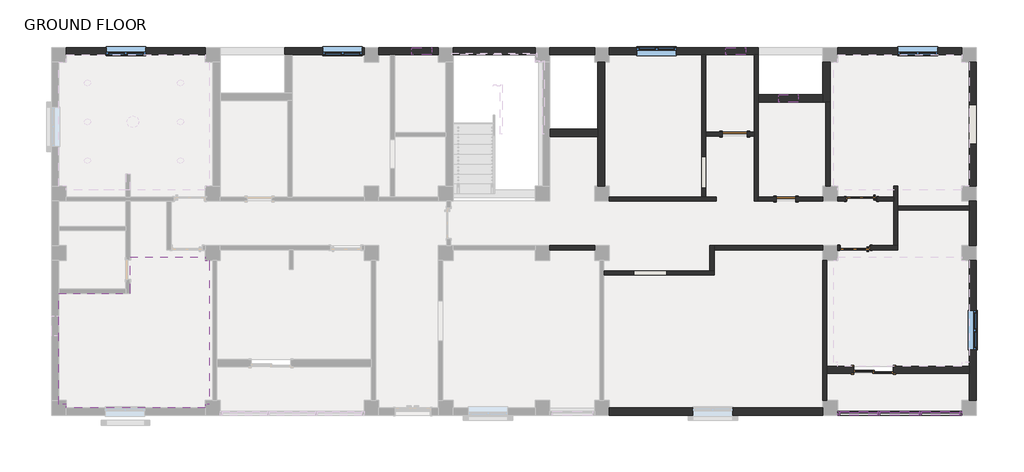
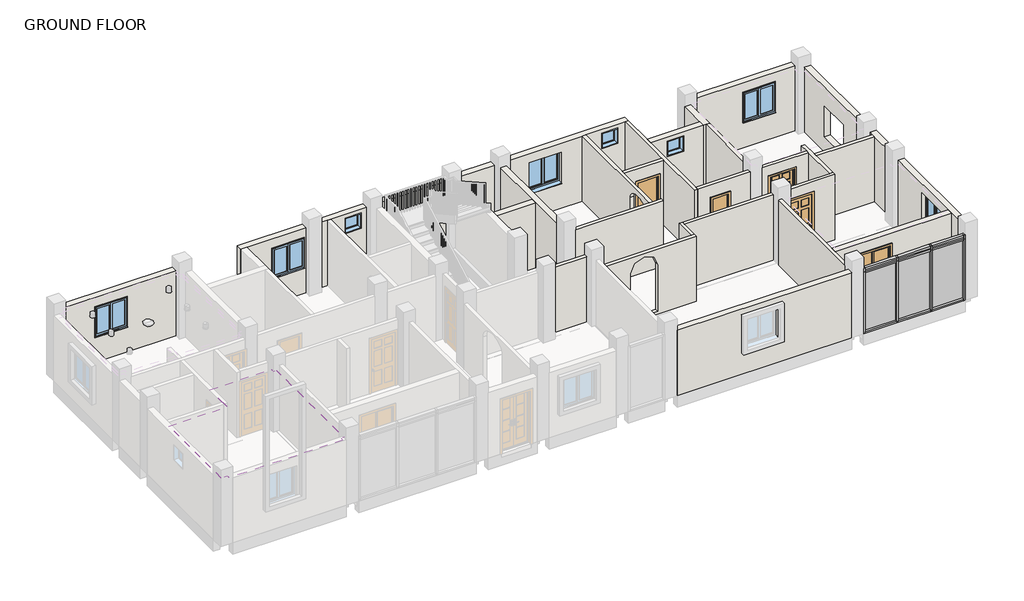
# One storey, part 2 of 5: 31 walls, 17 members, 8 windows, 6 plates, 5 doors, 1 covering.
"""IFC4 building model written with IfcOpenShell, lengths in millimetres."""

from ifc_helpers import new_model, si_unit, point, frame, origin, place, context, project, spatial, polyline, ellipse_curve, trimmed, outline, extrude, faceted_brep, transform, mapped, element, save
from ifc_brep_helpers import plane_surface, extruded_surface, advanced_brep
from components import door_double_sliding_4436dcad, door_c610b25b, door_03e3dfb5, single_flush_2_x_7_bath_room_door_025d1c86, door_1fe7f57d, member_5d96a33e, member_91edd790, member_f0fea5a5, member_f6f0dfdd, member_ee409385, member_876f8f00, member_7f2c8287, member_abd5b11f, system_panel_glazed_688a88ce, system_panel_glazed_153d3200, system_panel_glazed_8661f242, system_panel_glazed_4956db27, window_80340324, w2_0001_4_x_4_window_9dec5fc7

model = new_model("IFC4")

# Units and contexts
model_context = context("Model", 3, world=origin())
ifc_project = project(units=[si_unit("LENGTHUNIT", "METRE", prefix="MILLI")], contexts=[model_context])

# Site, building, storey
site = spatial("IfcSite", under=ifc_project)
building = spatial("IfcBuilding", under=site)
storey = spatial("IfcBuildingStorey", under=building, Name="GROUND FLOOR", Elevation=304.8)

# Covering
placement = place(None, origin())
element("IfcCovering", 1, ObjectType="GWB on Mtl. Stud", at=placement, inside=storey, context=model_context, shape_type="SweptSolid", body=[
    extrude(outline(polyline([(-15145.3456086, -10773.5679047), (-15145.3456086, -7363.1659448), (-12959.7401855, -7363.1659448), (-12959.7401855, -6244.0794704), (-10649.5456086, -6244.0794704), (-10649.5456086, -6358.3794704), (-10535.2456086, -6358.3794704), (-10535.2456086, -6963.5679047), (-10535.2456086, -10773.5679047), (-10649.5456086, -10773.5679047), (-10649.5456086, -10887.8679047), (-12959.7401855, -10887.8679047), (-14916.7456086, -10887.8679047), (-14916.7456086, -10773.5679047), (-15145.3456086, -10773.5679047)]), holes=[polyline([(-14840.5456086, -10583.0679047), (-10840.0456086, -10583.0679047), (-10840.0456086, -6548.8794704), (-12654.9401855, -6548.8794704), (-12654.9401855, -7667.9659448), (-14840.5456086, -7667.9659448), (-14840.5456086, -10583.0679047)])]), frame((0.0, 0.0, 2743.2), z_axis=(0.0, 0.0, 1.0), x_axis=(1.0, 0.0, 0.0)), (0.0, 0.0, 1.0), 107.95),
    extrude(outline(polyline([(-14688.1456086, -10430.6679047), (-14688.1456086, -7820.3659448), (-12502.5401855, -7820.3659448), (-12502.5401855, -6701.2794704), (-10992.4456086, -6701.2794704), (-10992.4456086, -10430.6679047), (-14688.1456086, -10430.6679047)]), holes=[polyline([(-14535.7456086, -7972.7659448), (-14535.7456086, -10278.2679047), (-11144.8456086, -10278.2679047), (-11144.8456086, -6853.6794704), (-12350.1401855, -6853.6794704), (-12350.1401855, -7972.7659448), (-14535.7456086, -7972.7659448)])]), frame((0.0, 0.0, 2743.2), z_axis=(0.0, 0.0, 1.0), x_axis=(1.0, 0.0, 0.0)), (0.0, 0.0, 1.0), 107.95),
])

# Doors
door_double_sliding_shape = door_double_sliding_4436dcad(model_context)
element("IfcDoor", 2, ObjectType="Door-Double-Sliding", at=placement, inside=storey, context=model_context, shape_type="MappedRepresentation", body=[
    mapped(door_double_sliding_shape, transform((9879.3128058, -9592.4679047, 304.8), x_axis=(-1.0, 0.0, 0.0), y_axis=(0.0, -1.0, 0.0), z_axis=(0.0, 0.0, 1.0))),
])
door_shape = door_c610b25b(model_context)
element("IfcDoor", 3, ObjectType="Door-Interior-Single-6_Panel-Wood : 36\" x 84\"", at=placement, inside=storey, context=model_context, shape_type="MappedRepresentation", body=[
    mapped(door_shape, transform((9511.0128058, -4462.9044704, 304.8), x_axis=(-1.0, 0.0, 0.0), y_axis=(0.0, -1.0, 0.0), z_axis=(0.0, 0.0, 1.0))),
])
door_2_shape = door_03e3dfb5(model_context)
element("IfcDoor", 4, ObjectType="Door-Interior-Single-6_Panel-Wood : 36\" x 84\"", at=placement, inside=storey, context=model_context, shape_type="MappedRepresentation", body=[
    mapped(door_2_shape, transform((9307.8128058, -5967.8544704, 304.8), x_axis=(-1.0, 0.0, 0.0), y_axis=(0.0, -1.0, 0.0), z_axis=(0.0, 0.0, 1.0))),
])
single_flush_2_x_7_bath_room_door_shape = single_flush_2_x_7_bath_room_door_025d1c86(model_context)
element("IfcDoor", 5, ObjectType="Single-Flush : 2' X 7' BATH ROOM DOOR", at=placement, inside=storey, context=model_context, shape_type="MappedRepresentation", body=[
    mapped(single_flush_2_x_7_bath_room_door_shape, transform((7190.4916602, -4466.0794704, 304.8), x_axis=(1.0, 0.0, 0.0), y_axis=(0.0, 1.0, 0.0), z_axis=(0.0, 0.0, 1.0))),
])
door_3_shape = door_1fe7f57d(model_context)
element("IfcDoor", 6, ObjectType="Single-Flush : 30\" x 80\"", at=placement, inside=storey, context=model_context, shape_type="MappedRepresentation", body=[
    mapped(door_3_shape, transform((5615.6916602, -2472.1794704, 304.8), x_axis=(1.0, 0.0, 0.0), y_axis=(0.0, 1.0, 0.0), z_axis=(0.0, 0.0, 1.0))),
])

# Members
member_shape = member_5d96a33e(model_context)
element("IfcMember", 7, ObjectType="Rectangular Mullion : 2.5\" x 5\" rectangular", at=placement, inside=storey, context=model_context, shape_type="MappedRepresentation", body=[
    mapped(member_shape, transform((12520.9128058, -11052.9679047, 2895.6), x_axis=(0.0, 0.0, 1.0), y_axis=(0.0, -1.0, 0.0), z_axis=(1.0, 0.0, 0.0))),
])
element("IfcMember", 8, ObjectType="Rectangular Mullion : 2.5\" x 5\" rectangular", at=placement, inside=storey, context=model_context, shape_type="MappedRepresentation", body=[
    mapped(member_shape, transform((10012.6628059, -11052.9679047, 2895.6), x_axis=(0.0, 0.0, 1.0), y_axis=(0.0, -1.0, 0.0), z_axis=(1.0, 0.0, 0.0))),
])
element("IfcMember", 9, ObjectType="Rectangular Mullion : 2.5\" x 5\" rectangular", at=placement, inside=storey, context=model_context, shape_type="MappedRepresentation", body=[
    mapped(member_shape, transform((8837.9128058, -11052.9679047, 304.8), x_axis=(0.0, 0.0, -1.0), y_axis=(0.0, -1.0, 0.0), z_axis=(-1.0, 0.0, 0.0))),
])
element("IfcMember", 10, ObjectType="Rectangular Mullion : 2.5\" x 5\" rectangular", at=placement, inside=storey, context=model_context, shape_type="MappedRepresentation", body=[
    mapped(member_shape, transform((11346.1628057, -11052.9679047, 304.8), x_axis=(0.0, 0.0, -1.0), y_axis=(0.0, -1.0, 0.0), z_axis=(-1.0, 0.0, 0.0))),
])
member_2_shape = member_91edd790(model_context)
element("IfcMember", 11, ObjectType="Rectangular Mullion : 2.5\" x 5\" rectangular", at=placement, inside=storey, context=model_context, shape_type="MappedRepresentation", body=[
    mapped(member_2_shape, transform((11282.6628057, -11052.9679047, 2895.6), x_axis=(0.0, 0.0, 1.0), y_axis=(0.0, -1.0, 0.0), z_axis=(1.0, 0.0, 0.0))),
])
element("IfcMember", 12, ObjectType="Rectangular Mullion : 2.5\" x 5\" rectangular", at=placement, inside=storey, context=model_context, shape_type="MappedRepresentation", body=[
    mapped(member_2_shape, transform((10076.1628059, -11052.9679047, 304.8), x_axis=(0.0, 0.0, -1.0), y_axis=(0.0, -1.0, 0.0), z_axis=(-1.0, 0.0, 0.0))),
])
member_3_shape = member_f0fea5a5(model_context)
element("IfcMember", 13, ObjectType="Rectangular Mullion : 2.5\" x 5\" rectangular", at=placement, inside=storey, context=model_context, shape_type="MappedRepresentation", body=[
    mapped(member_3_shape, transform((10044.4128059, -11052.9679047, 304.8), x_axis=(1.0, 0.0, 0.0), y_axis=(0.0, -1.0, 0.0), z_axis=(0.0, 0.0, -1.0))),
])
element("IfcMember", 14, ObjectType="Rectangular Mullion : 2.5\" x 5\" rectangular", at=placement, inside=storey, context=model_context, shape_type="MappedRepresentation", body=[
    mapped(member_3_shape, transform((11314.4128057, -11052.9679047, 304.8), x_axis=(1.0, 0.0, 0.0), y_axis=(0.0, -1.0, 0.0), z_axis=(0.0, 0.0, -1.0))),
])
member_4_shape = member_f6f0dfdd(model_context)
element("IfcMember", 15, ObjectType="Rectangular Mullion : 2.5\" x 5\" rectangular", at=placement, inside=storey, context=model_context, shape_type="MappedRepresentation", body=[
    mapped(member_4_shape, transform((10044.4128059, -11052.9679047, 2743.2), x_axis=(1.0, 0.0, 0.0), y_axis=(0.0, -1.0, 0.0), z_axis=(0.0, 0.0, -1.0))),
])
element("IfcMember", 16, ObjectType="Rectangular Mullion : 2.5\" x 5\" rectangular", at=placement, inside=storey, context=model_context, shape_type="MappedRepresentation", body=[
    mapped(member_4_shape, transform((11314.4128057, -11052.9679047, 2743.2), x_axis=(1.0, 0.0, 0.0), y_axis=(0.0, -1.0, 0.0), z_axis=(0.0, 0.0, -1.0))),
])
member_5_shape = member_ee409385(model_context)
element("IfcMember", 17, ObjectType="Rectangular Mullion : 2.5\" x 5\" rectangular", at=placement, inside=storey, context=model_context, shape_type="MappedRepresentation", body=[
    mapped(member_5_shape, transform((12584.4128058, -11052.9679047, 304.8), x_axis=(1.0, 0.0, 0.0), y_axis=(0.0, -1.0, 0.0), z_axis=(0.0, 0.0, -1.0))),
])
member_6_shape = member_876f8f00(model_context)
element("IfcMember", 18, ObjectType="Rectangular Mullion : 2.5\" x 5\" rectangular", at=placement, inside=storey, context=model_context, shape_type="MappedRepresentation", body=[
    mapped(member_6_shape, transform((8774.4128058, -11052.9679047, 2895.6), x_axis=(-1.0, 0.0, 0.0), y_axis=(0.0, -1.0, 0.0), z_axis=(0.0, 0.0, 1.0))),
])
element("IfcMember", 19, ObjectType="Rectangular Mullion : 2.5\" x 5\" rectangular", at=placement, inside=storey, context=model_context, shape_type="MappedRepresentation", body=[
    mapped(member_6_shape, transform((12584.4128058, -11052.9679047, 2743.2), x_axis=(1.0, 0.0, 0.0), y_axis=(0.0, -1.0, 0.0), z_axis=(0.0, 0.0, -1.0))),
])
element("IfcMember", 20, ObjectType="Rectangular Mullion : 2.5\" x 5\" rectangular", at=placement, inside=storey, context=model_context, shape_type="MappedRepresentation", body=[
    mapped(member_5_shape, transform((8774.4128058, -11052.9679047, 2743.2), x_axis=(-1.0, 0.0, 0.0), y_axis=(0.0, -1.0, 0.0), z_axis=(0.0, 0.0, 1.0))),
])
member_7_shape = member_7f2c8287(model_context)
element("IfcMember", 21, ObjectType="Rectangular Mullion : 2.5\" x 5\" rectangular", at=placement, inside=storey, context=model_context, shape_type="MappedRepresentation", body=[
    mapped(member_7_shape, transform((10012.6628059, -11052.9679047, 2743.2), x_axis=(0.0, 0.0, 1.0), y_axis=(0.0, -1.0, 0.0), z_axis=(1.0, 0.0, 0.0))),
])
element("IfcMember", 22, ObjectType="Rectangular Mullion : 2.5\" x 5\" rectangular", at=placement, inside=storey, context=model_context, shape_type="MappedRepresentation", body=[
    mapped(member_7_shape, transform((12520.9128058, -11052.9679047, 2743.2), x_axis=(0.0, 0.0, 1.0), y_axis=(0.0, -1.0, 0.0), z_axis=(1.0, 0.0, 0.0))),
])
member_8_shape = member_abd5b11f(model_context)
element("IfcMember", 23, ObjectType="Rectangular Mullion : 2.5\" x 5\" rectangular", at=placement, inside=storey, context=model_context, shape_type="MappedRepresentation", body=[
    mapped(member_8_shape, transform((11282.6628057, -11052.9679047, 2743.2), x_axis=(0.0, 0.0, 1.0), y_axis=(0.0, -1.0, 0.0), z_axis=(1.0, 0.0, 0.0))),
])

# Plates
system_panel_glazed_shape = system_panel_glazed_688a88ce(model_context)
element("IfcPlate", 24, ObjectType="System Panel : Glazed", at=placement, inside=storey, context=model_context, shape_type="MappedRepresentation", body=[
    mapped(system_panel_glazed_shape, transform((9425.2878058, -11052.9679047, 368.3), x_axis=(1.0, 0.0, 0.0), y_axis=(0.0, 1.0, 0.0), z_axis=(0.0, 0.0, 1.0))),
])
element("IfcPlate", 25, ObjectType="System Panel : Glazed", at=placement, inside=storey, context=model_context, shape_type="MappedRepresentation", body=[
    mapped(system_panel_glazed_shape, transform((11933.5378057, -11052.9679047, 368.3), x_axis=(1.0, 0.0, 0.0), y_axis=(0.0, 1.0, 0.0), z_axis=(0.0, 0.0, 1.0))),
])
system_panel_glazed_2_shape = system_panel_glazed_153d3200(model_context)
element("IfcPlate", 26, ObjectType="System Panel : Glazed", at=placement, inside=storey, context=model_context, shape_type="MappedRepresentation", body=[
    mapped(system_panel_glazed_2_shape, transform((10679.4128058, -11052.9679047, 368.3), x_axis=(1.0, 0.0, 0.0), y_axis=(0.0, 1.0, 0.0), z_axis=(0.0, 0.0, 1.0))),
])
system_panel_glazed_3_shape = system_panel_glazed_8661f242(model_context)
element("IfcPlate", 27, ObjectType="System Panel : Glazed", at=placement, inside=storey, context=model_context, shape_type="MappedRepresentation", body=[
    mapped(system_panel_glazed_3_shape, transform((9425.2878058, -11052.9679047, 2774.95), x_axis=(1.0, 0.0, 0.0), y_axis=(0.0, 1.0, 0.0), z_axis=(0.0, 0.0, 1.0))),
])
element("IfcPlate", 28, ObjectType="System Panel : Glazed", at=placement, inside=storey, context=model_context, shape_type="MappedRepresentation", body=[
    mapped(system_panel_glazed_3_shape, transform((11933.5378057, -11052.9679047, 2774.95), x_axis=(1.0, 0.0, 0.0), y_axis=(0.0, 1.0, 0.0), z_axis=(0.0, 0.0, 1.0))),
])
system_panel_glazed_4_shape = system_panel_glazed_4956db27(model_context)
element("IfcPlate", 29, ObjectType="System Panel : Glazed", at=placement, inside=storey, context=model_context, shape_type="MappedRepresentation", body=[
    mapped(system_panel_glazed_4_shape, transform((10679.4128058, -11052.9679047, 2774.95), x_axis=(1.0, 0.0, 0.0), y_axis=(0.0, 1.0, 0.0), z_axis=(0.0, 0.0, 1.0))),
])

# Walls
element("IfcWall", 30, ObjectType="EXTERIOR WALL 9\"", at=placement, inside=storey, context=model_context, shape_type="SweptSolid", body=[
    extrude(outline(polyline([(304.8, 1767.5916602), (304.8, 8317.2128058), (2895.6, 8317.2128058), (2895.6, 1767.5916602), (304.8, 1767.5916602)]), holes=[polyline([(1304.8, 5552.1916602), (1304.8, 4332.9916602), (2524.0, 4332.9916602), (2524.0, 5552.1916602), (1304.8, 5552.1916602)])]), frame((0.0, -11116.4679047, 0.0), z_axis=(0.0, 1.0, 0.0), x_axis=(0.0, 0.0, 1.0)), (0.0, 0.0, 1.0), 228.6),
])
element("IfcWall", 31, ObjectType="EXTERIOR WALL 9\"", at=placement, inside=storey, context=model_context, shape_type="Brep", body=[
    faceted_brep([(13041.6128058, -10659.2679047, 304.8), (13041.6128058, -6358.3794704, 304.8), (13041.6128058, -6358.3794704, 2895.6), (13041.6128058, -10659.2679047, 2895.6), (13041.6128058, -9109.8679047, 1304.8), (13041.6128058, -9109.8679047, 2524.0), (13041.6128058, -7890.6679047, 2524.0), (13041.6128058, -7890.6679047, 1304.8), (12813.0128058, -10659.2679047, 304.8), (12813.0128058, -10659.2679047, 2895.6), (12813.0128058, -9833.7679047, 2895.6), (12813.0128058, -9605.1679047, 2895.6), (12813.0128058, -6358.3794704, 2895.6), (12813.0128058, -6358.3794704, 304.8), (12813.0128058, -9605.1679047, 304.8), (12813.0128058, -9833.7679047, 304.8), (12813.0128058, -9109.8679047, 1304.8), (12813.0128058, -7890.6679047, 1304.8), (12813.0128058, -7890.6679047, 2524.0), (12813.0128058, -9109.8679047, 2524.0)], [[[0, 1, 2, 3], [4, 5, 6, 7]], [[8, 9, 10, 11, 12, 13, 14, 15], [16, 17, 18, 19]], [[1, 0, 8, 15, 14, 13]], [[2, 1, 13, 12]], [[3, 2, 12, 11, 10, 9]], [[0, 3, 9, 8]], [[5, 4, 16, 19]], [[6, 5, 19, 18]], [[7, 6, 18, 17]], [[4, 7, 17, 16]]]),
])
element("IfcWall", 32, ObjectType="EXTERIOR WALL 9\"", at=placement, inside=storey, context=model_context, shape_type="Brep", body=[
    faceted_brep([(13041.6128058, -5901.1794704, 304.8), (13041.6128058, -4529.5794704, 304.8), (13041.6128058, -4529.5794704, 2895.6), (13041.6128058, -5901.1794704, 2895.6), (12813.0128058, -5901.1794704, 304.8), (12813.0128058, -5901.1794704, 2895.6), (12813.0128058, -4808.9794704, 2895.6), (12813.0128058, -4681.9794704, 2895.6), (12813.0128058, -4529.5794704, 2895.6), (12813.0128058, -4529.5794704, 304.8), (12813.0128058, -4681.9794704, 304.8), (12813.0128058, -4808.9794704, 304.8)], [[[0, 1, 2, 3]], [[4, 5, 6, 7, 8, 9, 10, 11]], [[1, 0, 4, 11, 10, 9]], [[2, 1, 9, 8]], [[3, 2, 8, 7, 6, 5]], [[0, 3, 5, 4]]]),
])
element("IfcWall", 33, ObjectType="EXTERIOR WALL 9\"", at=placement, inside=storey, context=model_context, shape_type="SweptSolid", body=[
    extrude(outline(polyline([(-4072.3794704, 304.8), (-4072.3794704, 2895.6), (-262.3794704, 2895.6), (-262.3794704, 304.8), (-4072.3794704, 304.8)]), holes=[polyline([(-2776.9794704, 914.4), (-1557.7794704, 914.4), (-1557.7794704, 2133.6), (-2776.9794704, 2133.6), (-2776.9794704, 914.4)])]), frame((12813.0128058, 0.0, 0.0), z_axis=(1.0, 0.0, 0.0), x_axis=(0.0, 1.0, 0.0)), (0.0, 0.0, 1.0), 228.6),
])
element("IfcWall", 34, ObjectType="EXTERIOR WALL 9\"", at=placement, inside=storey, context=model_context, shape_type="SweptSolid", body=[
    extrude(outline(polyline([(304.8, 12584.4128058), (2895.6, 12584.4128058), (2895.6, 8774.4128058), (304.8, 8774.4128058), (304.8, 12584.4128058)]), holes=[polyline([(1304.8, 10628.6128058), (2524.0, 10628.6128058), (2524.0, 11847.8128058), (1304.8, 11847.8128058), (1304.8, 10628.6128058)])]), frame((0.0, -33.7794704, 0.0), z_axis=(0.0, 1.0, 0.0), x_axis=(0.0, 0.0, 1.0)), (0.0, 0.0, 1.0), 228.6),
])
element("IfcWall", 35, ObjectType="EXTERIOR WALL 9\"", at=placement, inside=storey, context=model_context, shape_type="SweptSolid", body=[
    extrude(outline(polyline([(304.8, -14916.7456086), (304.8, -10649.5456086), (2895.6, -10649.5456086), (2895.6, -14916.7456086), (304.8, -14916.7456086)]), holes=[polyline([(1304.8, -13697.5456086), (2524.0, -13697.5456086), (2524.0, -12478.3456086), (1304.8, -12478.3456086), (1304.8, -13697.5456086)])]), frame((0.0, -33.7794704, 0.0), z_axis=(0.0, 1.0, 0.0), x_axis=(0.0, 0.0, 1.0)), (0.0, 0.0, 1.0), 228.6),
])
element("IfcWall", 36, ObjectType="EXTERIOR WALL 9\"", at=placement, inside=storey, context=model_context, shape_type="SweptSolid", body=[
    extrude(outline(polyline([(304.8, 8444.2128058), (304.8, 9269.7128058), (2438.4, 9269.7128058), (2438.4, 10488.9128058), (304.8, 10488.9128058), (304.8, 12813.0128058), (2895.6, 12813.0128058), (2895.6, 8444.2128058), (304.8, 8444.2128058)])), frame((0.0, -9833.7679047, 0.0), z_axis=(0.0, 1.0, 0.0), x_axis=(0.0, 0.0, 1.0)), (0.0, 0.0, 1.0), 228.6),
])
element("IfcWall", 37, ObjectType="EXTERIOR WALL 9\"", at=placement, inside=storey, context=model_context, shape_type="Brep", body=[
    faceted_brep([(-5772.7456086, 194.8205296, 304.8), (-8211.1456086, 194.8205296, 304.8), (-8211.1456086, 194.8205296, 2895.6), (-5772.7456086, 194.8205296, 2895.6), (-7042.7456086, 194.8205296, 1304.8), (-5823.5456086, 194.8205296, 1304.8), (-5823.5456086, 194.8205296, 2524.0), (-7042.7456086, 194.8205296, 2524.0), (-5772.7456086, -33.7794704, 304.8), (-5772.7456086, -33.7794704, 2895.6), (-7982.5456086, -33.7794704, 2895.6), (-8211.1456086, -33.7794704, 2895.6), (-8211.1456086, -33.7794704, 304.8), (-7982.5456086, -33.7794704, 304.8), (-7042.7456086, -33.7794704, 1304.8), (-7042.7456086, -33.7794704, 2524.0), (-5823.5456086, -33.7794704, 2524.0), (-5823.5456086, -33.7794704, 1304.8)], [[[0, 1, 2, 3], [4, 5, 6, 7]], [[8, 9, 10, 11, 12, 13], [14, 15, 16, 17]], [[1, 0, 8, 13, 12]], [[3, 2, 11, 10, 9]], [[0, 3, 9, 8]], [[2, 1, 12, 11]], [[15, 14, 4, 7]], [[16, 15, 7, 6]], [[17, 16, 6, 5]], [[14, 17, 5, 4]]]),
])
element("IfcWall", 38, ObjectType="EXTERIOR WALL 9\"", at=placement, inside=storey, context=model_context, shape_type="Brep", body=[
    faceted_brep([(-5315.5456086, -33.7794704, 304.8), (-4959.9456086, -33.7794704, 304.8), (-4832.9456086, -33.7794704, 304.8), (-3486.7456086, -33.7794704, 304.8), (-3486.7456086, -33.7794704, 2895.6), (-4832.9456086, -33.7794704, 2895.6), (-4959.9456086, -33.7794704, 2895.6), (-5315.5456086, -33.7794704, 2895.6), (-3689.9456086, -33.7794704, 2743.2), (-3689.9456086, -33.7794704, 2133.6), (-4299.5456086, -33.7794704, 2133.6), (-4299.5456086, -33.7794704, 2743.2), (-3486.7456086, 194.8205296, 304.8), (-5315.5456086, 194.8205296, 304.8), (-5315.5456086, 194.8205296, 2895.6), (-3486.7456086, 194.8205296, 2895.6), (-3689.9456086, 194.8205296, 2133.6), (-3689.9456086, 194.8205296, 2743.2), (-4299.5456086, 194.8205296, 2743.2), (-4299.5456086, 194.8205296, 2133.6)], [[[0, 1, 2, 3, 4, 5, 6, 7], [8, 9, 10, 11]], [[12, 13, 14, 15], [16, 17, 18, 19]], [[3, 2, 1, 0, 13, 12]], [[4, 3, 12, 15]], [[7, 6, 5, 4, 15, 14]], [[0, 7, 14, 13]], [[8, 17, 16, 9]], [[9, 16, 19, 10]], [[10, 19, 18, 11]], [[17, 8, 11, 18]]]),
])
element("IfcWall", 39, ObjectType="EXTERIOR WALL 9\"", at=placement, inside=storey, context=model_context, shape_type="SweptSolid", body=[
    extrude(outline(polyline([(-518.4083398, -33.7794704), (-3029.5456086, -33.7794704), (-3029.5456086, 194.8205296), (-518.4083398, 194.8205296), (-518.4083398, -33.7794704)])), frame((0.0, 0.0, 304.8), z_axis=(0.0, 0.0, 1.0), x_axis=(1.0, 0.0, 0.0)), (0.0, 0.0, 1.0), 2590.8),
])
element("IfcWall", 40, ObjectType="EXTERIOR WALL 9\"", at=placement, inside=storey, context=model_context, shape_type="SweptSolid", body=[
    extrude(outline(polyline([(1310.3916602, -33.7794704), (-61.2083398, -33.7794704), (-61.2083398, 194.8205296), (1310.3916602, 194.8205296), (1310.3916602, -33.7794704)])), frame((0.0, 0.0, 304.8), z_axis=(0.0, 0.0, 1.0), x_axis=(1.0, 0.0, 0.0)), (0.0, 0.0, 1.0), 2590.8),
])
element("IfcWall", 41, ObjectType="EXTERIOR WALL 9\"", at=placement, inside=storey, context=model_context, shape_type="Brep", body=[
    faceted_brep([(1767.5916602, -33.7794704, 304.8), (4599.6916602, -33.7794704, 304.8), (4726.6916602, -33.7794704, 304.8), (6212.5916602, -33.7794704, 304.8), (6339.5916602, -33.7794704, 304.8), (6339.5916602, -33.7794704, 2895.6), (6212.5916602, -33.7794704, 2895.6), (4726.6916602, -33.7794704, 2895.6), (4599.6916602, -33.7794704, 2895.6), (1767.5916602, -33.7794704, 2895.6), (3824.9916602, -33.7794704, 1304.8), (2605.7916602, -33.7794704, 1304.8), (2605.7916602, -33.7794704, 2524.0), (3824.9916602, -33.7794704, 2524.0), (5945.8916602, -33.7794704, 2743.2), (5945.8916602, -33.7794704, 2133.6), (5336.2916602, -33.7794704, 2133.6), (5336.2916602, -33.7794704, 2743.2), (6339.5916602, 194.8205296, 304.8), (1767.5916602, 194.8205296, 304.8), (1767.5916602, 194.8205296, 2895.6), (6339.5916602, 194.8205296, 2895.6), (3824.9916602, 194.8205296, 1304.8), (3824.9916602, 194.8205296, 2524.0), (2605.7916602, 194.8205296, 2524.0), (2605.7916602, 194.8205296, 1304.8), (5945.8916602, 194.8205296, 2133.6), (5945.8916602, 194.8205296, 2743.2), (5336.2916602, 194.8205296, 2743.2), (5336.2916602, 194.8205296, 2133.6)], [[[0, 1, 2, 3, 4, 5, 6, 7, 8, 9], [10, 11, 12, 13], [14, 15, 16, 17]], [[18, 19, 20, 21], [22, 23, 24, 25], [26, 27, 28, 29]], [[4, 3, 2, 1, 0, 19, 18]], [[9, 8, 7, 6, 5, 21, 20]], [[0, 9, 20, 19]], [[5, 4, 18, 21]], [[23, 22, 10, 13]], [[24, 23, 13, 12]], [[25, 24, 12, 11]], [[22, 25, 11, 10]], [[14, 27, 26, 15]], [[15, 26, 29, 16]], [[16, 29, 28, 17]], [[27, 14, 17, 28]]]),
])
element("IfcWall", 42, ObjectType="EXTERIOR WALL 9\"", at=placement, inside=storey, context=model_context, shape_type="Brep", body=[
    faceted_brep([(8317.2128058, -262.3794704, 304.8), (8317.2128058, -1252.9794704, 304.8), (8317.2128058, -1481.5794704, 304.8), (8317.2128058, -1481.5794704, 2895.6), (8317.2128058, -1252.9794704, 2895.6), (8317.2128058, -262.3794704, 2895.6), (8545.8128058, -262.3794704, 304.8), (8545.8128058, -262.3794704, 2895.6), (8545.8128058, -1481.5794704, 2895.6), (8545.8128058, -1481.5794704, 304.8), (8418.8128058, -1481.5794704, 304.8), (8418.8128058, -1481.5794704, 2895.6)], [[[0, 1, 2, 3, 4, 5]], [[6, 7, 8, 9]], [[2, 1, 0, 6, 9, 10]], [[5, 4, 3, 11, 8, 7]], [[0, 5, 7, 6]], [[3, 2, 10, 9, 8, 11]]]),
])
element("IfcWall", 43, ObjectType="EXTERIOR WALL 9\"", at=placement, inside=storey, context=model_context, shape_type="SweptSolid", body=[
    extrude(outline(polyline([(304.8, 6339.5916602), (304.8, 8317.2128058), (2895.6, 8317.2128058), (2895.6, 6339.5916602), (304.8, 6339.5916602)]), holes=[polyline([(2743.2, 7571.4916602), (2133.6, 7571.4916602), (2133.6, 6961.8916602), (2743.2, 6961.8916602), (2743.2, 7571.4916602)])]), frame((0.0, -1481.5794704, 0.0), z_axis=(0.0, 1.0, 0.0), x_axis=(0.0, 0.0, 1.0)), (0.0, 0.0, 1.0), 228.6),
])
element("IfcWall", 44, ObjectType="EXTERIOR WALL 9\"", at=placement, inside=storey, context=model_context, shape_type="Brep", body=[
    faceted_brep([(1399.2916602, -262.3794704, 304.8), (1399.2916602, -2319.7794704, 304.8), (1399.2916602, -2548.3794704, 304.8), (1399.2916602, -4072.3794704, 304.8), (1399.2916602, -4072.3794704, 2895.6), (1399.2916602, -2548.3794704, 2895.6), (1399.2916602, -2319.7794704, 2895.6), (1399.2916602, -262.3794704, 2895.6), (1627.8916602, -262.3794704, 304.8), (1627.8916602, -262.3794704, 2895.6), (1627.8916602, -4072.3794704, 2895.6), (1627.8916602, -4072.3794704, 304.8)], [[[0, 1, 2, 3, 4, 5, 6, 7]], [[8, 9, 10, 11]], [[3, 2, 1, 0, 8, 11]], [[4, 3, 11, 10]], [[7, 6, 5, 4, 10, 9]], [[0, 7, 9, 8]]]),
])
element("IfcWall", 45, ObjectType="EXTERIOR WALL 9\"", at=placement, inside=storey, context=model_context, shape_type="SweptSolid", body=[
    extrude(outline(polyline([(1399.2916602, -2548.3794704), (-61.2083398, -2548.3794704), (-61.2083398, -2319.7794704), (1399.2916602, -2319.7794704), (1399.2916602, -2548.3794704)])), frame((0.0, 0.0, 304.8), z_axis=(0.0, 0.0, 1.0), x_axis=(1.0, 0.0, 0.0)), (0.0, 0.0, 1.0), 2590.8),
])
element("IfcWall", 46, ObjectType="INTERIOR WALL 5\"", at=placement, inside=storey, context=model_context, shape_type="Brep", body=[
    faceted_brep([(8444.2128058, -10659.2679047, 304.8), (8444.2128058, -9833.7679047, 304.8), (8444.2128058, -9605.1679047, 304.8), (8444.2128058, -6358.3794704, 304.8), (8444.2128058, -6358.3794704, 2895.6), (8444.2128058, -9605.1679047, 2895.6), (8444.2128058, -9833.7679047, 2895.6), (8444.2128058, -10659.2679047, 2895.6), (8317.2128058, -10659.2679047, 304.8), (8317.2128058, -10659.2679047, 2895.6), (8317.2128058, -6358.3794704, 2895.6), (8317.2128058, -6358.3794704, 304.8)], [[[0, 1, 2, 3, 4, 5, 6, 7]], [[8, 9, 10, 11]], [[3, 2, 1, 0, 8, 11]], [[4, 3, 11, 10]], [[7, 6, 5, 4, 10, 9]], [[0, 7, 9, 8]]]),
])
element("IfcWall", 47, ObjectType="INTERIOR WALL 5\"", at=placement, inside=storey, context=model_context, shape_type="SweptSolid", body=[
    extrude(outline(polyline([(10628.6128058, -4681.9794704), (12813.0128058, -4681.9794704), (12813.0128058, -4808.9794704), (10628.6128058, -4808.9794704), (10628.6128058, -4681.9794704)])), frame((0.0, 0.0, 304.8), z_axis=(0.0, 0.0, 1.0), x_axis=(1.0, 0.0, 0.0)), (0.0, 0.0, 1.0), 2590.8),
])
element("IfcWall", 48, ObjectType="INTERIOR WALL 5\"", at=placement, inside=storey, context=model_context, shape_type="Brep", body=[
    faceted_brep([(10628.6128058, -6028.1794704, 2895.6), (8774.4128058, -6028.1794704, 2895.6), (8774.4128058, -6028.1794704, 304.8), (8825.2128058, -6028.1794704, 304.8), (8825.2128058, -6028.1794704, 2463.8), (9790.4128058, -6028.1794704, 2463.8), (9790.4128058, -6028.1794704, 304.8), (10628.6128058, -6028.1794704, 304.8), (8774.4128058, -5901.1794704, 2895.6), (10501.6128058, -5901.1794704, 2895.6), (10628.6128058, -5901.1794704, 2895.6), (10628.6128058, -5901.1794704, 304.8), (10501.6128058, -5901.1794704, 304.8), (9790.4128058, -5901.1794704, 304.8), (9790.4128058, -5901.1794704, 2463.8), (8825.2128058, -5901.1794704, 2463.8), (8825.2128058, -5901.1794704, 304.8), (8774.4128058, -5901.1794704, 304.8)], [[[0, 1, 2, 3, 4, 5, 6, 7]], [[8, 9, 10, 11, 12, 13, 14, 15, 16, 17]], [[2, 17, 16, 3]], [[11, 7, 6, 13, 12]], [[1, 0, 10, 9, 8]], [[2, 1, 8, 17]], [[0, 7, 11, 10]], [[15, 4, 3, 16]], [[4, 15, 14, 5]], [[5, 14, 13, 6]]]),
])
element("IfcWall", 49, ObjectType="INTERIOR WALL 5\"", at=placement, inside=storey, context=model_context, shape_type="Brep", body=[
    faceted_brep([(10628.6128058, -5901.1794704, 304.8), (10628.6128058, -4808.9794704, 304.8), (10628.6128058, -4681.9794704, 304.8), (10628.6128058, -4072.3794704, 304.8), (10628.6128058, -4072.3794704, 2895.6), (10628.6128058, -4681.9794704, 2895.6), (10628.6128058, -4808.9794704, 2895.6), (10628.6128058, -5901.1794704, 2895.6), (10501.6128058, -5901.1794704, 304.8), (10501.6128058, -5901.1794704, 2895.6), (10501.6128058, -4529.5794704, 2895.6), (10501.6128058, -4402.5794704, 2895.6), (10501.6128058, -4072.3794704, 2895.6), (10501.6128058, -4072.3794704, 304.8), (10501.6128058, -4402.5794704, 304.8), (10501.6128058, -4529.5794704, 304.8)], [[[0, 1, 2, 3, 4, 5, 6, 7]], [[8, 9, 10, 11, 12, 13, 14, 15]], [[3, 2, 1, 0, 8, 15, 14, 13]], [[4, 3, 13, 12]], [[7, 6, 5, 4, 12, 11, 10, 9]], [[0, 7, 9, 8]]]),
])
element("IfcWall", 50, ObjectType="INTERIOR WALL 5\"", at=placement, inside=storey, context=model_context, shape_type="Brep", body=[
    faceted_brep([(6212.5916602, -33.7794704, 304.8), (6212.5916602, -2408.6794704, 304.8), (6212.5916602, -2535.6794704, 304.8), (6212.5916602, -4529.5794704, 304.8), (6212.5916602, -4529.5794704, 2895.6), (6212.5916602, -2535.6794704, 2895.6), (6212.5916602, -2408.6794704, 2895.6), (6212.5916602, -33.7794704, 2895.6), (6339.5916602, -33.7794704, 304.8), (6339.5916602, -33.7794704, 2895.6), (6339.5916602, -1252.9794704, 2895.6), (6339.5916602, -1481.5794704, 2895.6), (6339.5916602, -4402.5794704, 2895.6), (6339.5916602, -4529.5794704, 2895.6), (6339.5916602, -4529.5794704, 304.8), (6339.5916602, -4402.5794704, 304.8), (6339.5916602, -1481.5794704, 304.8), (6339.5916602, -1252.9794704, 304.8)], [[[0, 1, 2, 3, 4, 5, 6, 7]], [[8, 9, 10, 11, 12, 13, 14, 15, 16, 17]], [[3, 2, 1, 0, 8, 17, 16, 15, 14]], [[7, 6, 5, 4, 13, 12, 11, 10, 9]], [[0, 7, 9, 8]], [[4, 3, 14, 13]]]),
])
element("IfcWall", 51, ObjectType="INTERIOR WALL 5\"", at=placement, inside=storey, context=model_context, shape_type="SweptSolid", body=[
    extrude(outline(polyline([(8418.8128058, -4072.3794704), (8418.8128058, -1481.5794704), (8545.8128058, -1481.5794704), (8545.8128058, -4072.3794704), (8418.8128058, -4072.3794704)])), frame((0.0, 0.0, 304.8), z_axis=(0.0, 0.0, 1.0), x_axis=(1.0, 0.0, 0.0)), (0.0, 0.0, 1.0), 2590.8),
])
element("IfcWall", 52, ObjectType="INTERIOR WALL 5\"", at=placement, inside=storey, context=model_context, shape_type="Brep", body=[
    faceted_brep([(1767.5916602, -4529.5794704, 304.8), (5044.1916602, -4529.5794704, 304.8), (5044.1916602, -4529.5794704, 2895.6), (1767.5916602, -4529.5794704, 2895.6), (1767.5916602, -4402.5794704, 304.8), (1767.5916602, -4402.5794704, 2895.6), (4599.6916602, -4402.5794704, 2895.6), (4726.6916602, -4402.5794704, 2895.6), (5044.1916602, -4402.5794704, 2895.6), (5044.1916602, -4402.5794704, 304.8), (4726.6916602, -4402.5794704, 304.8), (4599.6916602, -4402.5794704, 304.8)], [[[0, 1, 2, 3]], [[4, 5, 6, 7, 8, 9, 10, 11]], [[1, 0, 4, 11, 10, 9]], [[2, 1, 9, 8]], [[3, 2, 8, 7, 6, 5]], [[0, 3, 5, 4]]]),
])
element("IfcWall", 53, ObjectType="INTERIOR WALL 5\"", at=placement, inside=storey, context=model_context, shape_type="AdvancedBrep", body=[
    advanced_brep(
    [(4599.6916602, -33.7794704, 304.8), (4599.6916602, -4402.5794704, 304.8), (4599.6916602, -4402.5794704, 2895.6), (4599.6916602, -33.7794704, 2895.6), (4599.6916602, -3162.9760679, 2363.4701015), (4599.6916602, -4128.1760679, 2363.4701015), (4599.6916602, -4128.1760679, 483.8701015), (4599.6916602, -3162.9760679, 483.8701015), (4726.6916602, -33.7794704, 304.8), (4726.6916602, -33.7794704, 2895.6), (4726.6916602, -2408.6794704, 2895.6), (4726.6916602, -2535.6794704, 2895.6), (4726.6916602, -4402.5794704, 2895.6), (4726.6916602, -4402.5794704, 304.8), (4726.6916602, -2535.6794704, 304.8), (4726.6916602, -2408.6794704, 304.8), (4726.6916602, -3162.9760679, 2363.4701015), (4726.6916602, -3162.9760679, 483.8701015), (4726.6916602, -4128.1760679, 483.8701015), (4726.6916602, -4128.1760679, 2363.4701015)],
    [
        (0, 1),
        (1, 2),
        (2, 3),
        (3, 0),
        (4, 5, ellipse_curve(frame((4599.6916602, -3645.5760679, 2363.4701015), z_axis=(1.0, 0.0, 0.0), x_axis=(0.0, -1.0, 0.0)), 482.6, 330.2)),
        (5, 6),
        (6, 7),
        (7, 4),
        (8, 9),
        (9, 10),
        (10, 11),
        (11, 12),
        (12, 13),
        (13, 14),
        (14, 15),
        (15, 8),
        (16, 17),
        (17, 18),
        (18, 19),
        (19, 16, ellipse_curve(frame((4726.6916602, -3645.5760679, 2363.4701015), z_axis=(-1.0, 0.0, 0.0), x_axis=(0.0, -1.0, 0.0)), 482.6, 330.2)),
        (3, 9),
        (8, 0),
        (1, 13),
        (12, 2),
        (4, 16),
        (19, 5),
        (18, 6),
        (17, 7),
    ],
    [
        plane_surface(frame((4599.6916602, -33.7794704, 304.8), z_axis=(-1.0, 0.0, 0.0), x_axis=(0.0, -1.0, 0.0))),
        plane_surface(frame((4726.6916602, -33.7794704, 304.8), z_axis=(1.0, 0.0, 0.0), x_axis=(0.0, 1.0, 0.0))),
        plane_surface(frame((1784.6412895, -33.7794704, 304.8), z_axis=(0.0, 1.0, 0.0), x_axis=(1.0, 0.0, 0.0))),
        plane_surface(frame((1767.5916602, -4402.5794704, 304.8), z_axis=(0.0, -1.0, 0.0), x_axis=(-1.0, 0.0, 0.0))),
        plane_surface(frame((4599.6916602, 80.5205296, 304.8), z_axis=(0.0, 0.0, -1.0), x_axis=(1.0, 0.0, 0.0))),
        plane_surface(frame((4599.6916602, -4466.0794704, 2895.6), z_axis=(0.0, 0.0, 1.0), x_axis=(1.0, 0.0, 0.0))),
        extruded_surface(trimmed(ellipse_curve(frame((4790.1916602, -3645.5760679, 2363.4701015), z_axis=(1.0, 0.0, 0.0), x_axis=(0.0, -1.0, 0.0)), 482.6, 330.2), [point((4790.1916602, -3162.9760679, 2363.4701015))], [point((4790.1916602, -4128.1760679, 2363.4701015))], True, "CARTESIAN"), (-127.0, 0.0, 0.0), 127.0),
        plane_surface(frame((4599.6916602, -4128.1760679, 2363.4701015), z_axis=(0.0, 1.0, 0.0), x_axis=(1.0, 0.0, 0.0))),
        plane_surface(frame((4599.6916602, -4128.1760679, 483.8701015), z_axis=(0.0, 0.0, 1.0), x_axis=(1.0, 0.0, 0.0))),
        plane_surface(frame((4599.6916602, -3162.9760679, 483.8701015), z_axis=(0.0, -1.0, 0.0), x_axis=(1.0, 0.0, 0.0))),
    ],
    [
        (0, [[1, 2, 3, 4], [5, 6, 7, 8]]),
        (1, [[9, 10, 11, 12, 13, 14, 15, 16], [17, 18, 19, 20]]),
        (2, [[-4, 21, -9, 22]]),
        (3, [[-2, 23, -13, 24]]),
        (4, [[-1, -22, -16, -15, -14, -23]]),
        (5, [[-3, -24, -12, -11, -10, -21]]),
        (6, [[-5, 25, -20, 26]]),
        (7, [[-6, -26, -19, 27]]),
        (8, [[-7, -27, -18, 28]]),
        (9, [[-8, -28, -17, -25]]),
    ],
),
])
element("IfcWall", 54, ObjectType="INTERIOR WALL 5\"", at=placement, inside=storey, context=model_context, shape_type="SweptSolid", body=[
    extrude(outline(polyline([(2336.8, 5996.6916602), (304.8, 5996.6916602), (304.8, 6212.5916602), (2895.6, 6212.5916602), (2895.6, 4726.6916602), (304.8, 4726.6916602), (304.8, 5234.6916602), (2336.8, 5234.6916602), (2336.8, 5996.6916602)])), frame((0.0, -2535.6794704, 0.0), z_axis=(0.0, 1.0, 0.0), x_axis=(0.0, 0.0, 1.0)), (0.0, 0.0, 1.0), 127.0),
])
element("IfcWall", 55, ObjectType="INTERIOR WALL 5\"", at=placement, inside=storey, context=model_context, shape_type="SweptSolid", body=[
    extrude(outline(polyline([(2336.8, 7495.2916602), (304.8, 7495.2916602), (304.8, 8317.2128058), (2895.6, 8317.2128058), (2895.6, 6339.5916602), (304.8, 6339.5916602), (304.8, 6885.6916602), (2336.8, 6885.6916602), (2336.8, 7495.2916602)])), frame((0.0, -4529.5794704, 0.0), z_axis=(0.0, 1.0, 0.0), x_axis=(0.0, 0.0, 1.0)), (0.0, 0.0, 1.0), 127.0),
])
element("IfcWall", 56, ObjectType="INTERIOR WALL 5\"", at=placement, inside=storey, context=model_context, shape_type="SweptSolid", body=[
    extrude(outline(polyline([(2895.6, 10501.6128058), (2895.6, 8774.4128058), (304.8, 8774.4128058), (304.8, 9028.4128058), (2463.8, 9028.4128058), (2463.8, 9993.6128058), (304.8, 9993.6128058), (304.8, 10501.6128058), (2895.6, 10501.6128058)])), frame((0.0, -4529.5794704, 0.0), z_axis=(0.0, 1.0, 0.0), x_axis=(0.0, 0.0, 1.0)), (0.0, 0.0, 1.0), 127.0),
])
element("IfcWall", 57, ObjectType="INTERIOR WALL 5\"", at=placement, inside=storey, context=model_context, shape_type="SweptSolid", body=[
    extrude(outline(polyline([(-61.2083398, -5901.1794704), (1310.3916602, -5901.1794704), (1310.3916602, -6028.1794704), (-61.2083398, -6028.1794704), (-61.2083398, -5901.1794704)])), frame((0.0, 0.0, 304.8), z_axis=(0.0, 0.0, 1.0), x_axis=(1.0, 0.0, 0.0)), (0.0, 0.0, 1.0), 2590.8),
])
element("IfcWall", 58, ObjectType="INTERIOR WALL 5\"", at=placement, inside=storey, context=model_context, shape_type="AdvancedBrep", body=[
    advanced_brep(
    [(1589.7916602, -6802.8794704, 304.8), (4980.6916602, -6802.8794704, 304.8), (4980.6916602, -6802.8794704, 2895.6), (1589.7916602, -6802.8794704, 2895.6), (2514.6258025, -6802.8794704, 2267.5597277), (3530.6258025, -6802.8794704, 2267.5597277), (3530.6258025, -6802.8794704, 413.3597277), (2514.6258025, -6802.8794704, 413.3597277), (1589.7916602, -6675.8794704, 304.8), (1589.7916602, -6675.8794704, 2895.6), (4853.6916602, -6675.8794704, 2895.6), (4980.6916602, -6675.8794704, 2895.6), (4980.6916602, -6675.8794704, 304.8), (4853.6916602, -6675.8794704, 304.8), (2514.6258025, -6675.8794704, 2267.5597277), (2514.6258025, -6675.8794704, 413.3597277), (3530.6258025, -6675.8794704, 413.3597277), (3530.6258025, -6675.8794704, 2267.5597277)],
    [
        (0, 1),
        (1, 2),
        (2, 3),
        (3, 0),
        (4, 5, ellipse_curve(frame((3022.6258025, -6802.8794704, 2267.5597277), z_axis=(0.0, 1.0, 0.0), x_axis=(-1.0, 0.0, 0.0)), 508.0, 482.6)),
        (5, 6),
        (6, 7),
        (7, 4),
        (8, 9),
        (9, 10),
        (10, 11),
        (11, 12),
        (12, 13),
        (13, 8),
        (14, 15),
        (15, 16),
        (16, 17),
        (17, 14, ellipse_curve(frame((3022.6258025, -6675.8794704, 2267.5597277), z_axis=(0.0, -1.0, 0.0), x_axis=(-1.0, 0.0, 0.0)), 508.0, 482.6)),
        (3, 9),
        (8, 0),
        (1, 12),
        (11, 2),
        (4, 14),
        (17, 5),
        (16, 6),
        (15, 7),
    ],
    [
        plane_surface(frame((1589.7916602, -6802.8794704, 304.8), z_axis=(0.0, -1.0, 0.0), x_axis=(1.0, 0.0, 0.0))),
        plane_surface(frame((1589.7916602, -6675.8794704, 304.8), z_axis=(0.0, 1.0, 0.0), x_axis=(-1.0, 0.0, 0.0))),
        plane_surface(frame((1589.7916602, -10648.7570633, 304.8), z_axis=(-1.0, 0.0, 0.0), x_axis=(0.0, 1.0, 0.0))),
        plane_surface(frame((4980.6916602, -6675.8794704, 304.8), z_axis=(1.0, 0.0, 0.0), x_axis=(0.0, 1.0, 0.0))),
        plane_surface(frame((1526.2916602, -6802.8794704, 304.8), z_axis=(0.0, 0.0, -1.0), x_axis=(0.0, 1.0, 0.0))),
        plane_surface(frame((4917.1916602, -6802.8794704, 2895.6), z_axis=(0.0, 0.0, 1.0), x_axis=(0.0, 1.0, 0.0))),
        extruded_surface(trimmed(ellipse_curve(frame((3022.6258025, -6612.3794704, 2267.5597277), z_axis=(0.0, 1.0, 0.0), x_axis=(-1.0, 0.0, 0.0)), 508.0, 482.6), [point((2514.6258025, -6612.3794704, 2267.5597277))], [point((3530.6258025, -6612.3794704, 2267.5597277))], True, "CARTESIAN"), (0.0, -127.0, 0.0), 127.0),
        plane_surface(frame((3530.6258025, -6802.8794704, 2267.5597277), z_axis=(-1.0, 0.0, 0.0), x_axis=(0.0, 1.0, 0.0))),
        plane_surface(frame((3530.6258025, -6802.8794704, 413.3597277), z_axis=(0.0, 0.0, 1.0), x_axis=(0.0, 1.0, 0.0))),
        plane_surface(frame((2514.6258025, -6802.8794704, 413.3597277), z_axis=(1.0, 0.0, 0.0), x_axis=(0.0, 1.0, 0.0))),
    ],
    [
        (0, [[1, 2, 3, 4], [5, 6, 7, 8]]),
        (1, [[9, 10, 11, 12, 13, 14], [15, 16, 17, 18]]),
        (2, [[-4, 19, -9, 20]]),
        (3, [[-2, 21, -12, 22]]),
        (4, [[-1, -20, -14, -13, -21]]),
        (5, [[-3, -22, -11, -10, -19]]),
        (6, [[-5, 23, -18, 24]]),
        (7, [[-6, -24, -17, 25]]),
        (8, [[-7, -25, -16, 26]]),
        (9, [[-8, -26, -15, -23]]),
    ],
),
])
element("IfcWall", 59, ObjectType="INTERIOR WALL 5\"", at=placement, inside=storey, context=model_context, shape_type="Brep", body=[
    faceted_brep([(4980.6916602, -6675.8794704, 304.8), (4980.6916602, -6028.1794704, 304.8), (4980.6916602, -5901.1794704, 304.8), (4980.6916602, -5901.1794704, 2895.6), (4980.6916602, -6028.1794704, 2895.6), (4980.6916602, -6675.8794704, 2895.6), (4853.6916602, -6675.8794704, 304.8), (4853.6916602, -6675.8794704, 2895.6), (4853.6916602, -5901.1794704, 2895.6), (4853.6916602, -5901.1794704, 304.8)], [[[0, 1, 2, 3, 4, 5]], [[6, 7, 8, 9]], [[2, 1, 0, 6, 9]], [[5, 4, 3, 8, 7]], [[0, 5, 7, 6]], [[3, 2, 9, 8]]]),
])
element("IfcWall", 60, ObjectType="INTERIOR WALL 5\"", at=placement, inside=storey, context=model_context, shape_type="SweptSolid", body=[
    extrude(outline(polyline([(4980.6916602, -5901.1794704), (8317.2128058, -5901.1794704), (8317.2128058, -6028.1794704), (4980.6916602, -6028.1794704), (4980.6916602, -5901.1794704)])), frame((0.0, 0.0, 304.8), z_axis=(0.0, 0.0, 1.0), x_axis=(1.0, 0.0, 0.0)), (0.0, 0.0, 1.0), 2590.8),
])

# Windows
window_shape = window_80340324(model_context)
element("IfcWindow", 61, ObjectType="Fixed : 24\" x 24\"", at=placement, inside=storey, context=model_context, shape_type="MappedRepresentation", body=[
    mapped(window_shape, transform((-3956.6456086, 80.5205296, 1219.2), x_axis=(1.0, 0.0, 0.0), y_axis=(0.0, 1.0, 0.0), z_axis=(0.0, 0.0, 1.0))),
])
element("IfcWindow", 62, ObjectType="Fixed : 24\" x 24\"", at=placement, inside=storey, context=model_context, shape_type="MappedRepresentation", body=[
    mapped(window_shape, transform((7304.7916602, -1367.2794704, 1219.2), x_axis=(1.0, 0.0, 0.0), y_axis=(0.0, 1.0, 0.0), z_axis=(0.0, 0.0, 1.0))),
])
element("IfcWindow", 63, ObjectType="Fixed : 24\" x 24\"", at=placement, inside=storey, context=model_context, shape_type="MappedRepresentation", body=[
    mapped(window_shape, transform((5679.1916602, 80.5205296, 1219.2), x_axis=(1.0, 0.0, 0.0), y_axis=(0.0, 1.0, 0.0), z_axis=(0.0, 0.0, 1.0))),
])
w2_0001_4_x_4_window_shape = w2_0001_4_x_4_window_9dec5fc7(model_context)
element("IfcWindow", 64, ObjectType="w2.0001 : 4' X 4' WINDOW", at=placement, inside=storey, context=model_context, shape_type="MappedRepresentation", body=[
    mapped(w2_0001_4_x_4_window_shape, transform((11238.2128058, 80.5205296, 304.8), x_axis=(1.0, 0.0, 0.0), y_axis=(0.0, 1.0, 0.0), z_axis=(0.0, 0.0, 1.0))),
])
element("IfcWindow", 65, ObjectType="w2.0001 : 4' X 4' WINDOW", at=placement, inside=storey, context=model_context, shape_type="MappedRepresentation", body=[
    mapped(w2_0001_4_x_4_window_shape, transform((3215.3916602, 80.5205296, 304.8), x_axis=(-1.0, 0.0, 0.0), y_axis=(0.0, -1.0, 0.0), z_axis=(0.0, 0.0, 1.0))),
])
element("IfcWindow", 66, ObjectType="w2.0001 : 4' X 4' WINDOW", at=placement, inside=storey, context=model_context, shape_type="MappedRepresentation", body=[
    mapped(w2_0001_4_x_4_window_shape, transform((-6433.1456086, 80.5205296, 304.8), x_axis=(1.0, 0.0, 0.0), y_axis=(0.0, 1.0, 0.0), z_axis=(0.0, 0.0, 1.0))),
])
element("IfcWindow", 67, ObjectType="w2.0001 : 4' X 4' WINDOW", at=placement, inside=storey, context=model_context, shape_type="MappedRepresentation", body=[
    mapped(w2_0001_4_x_4_window_shape, transform((-13087.9456086, 80.5205296, 304.8), x_axis=(1.0, 0.0, 0.0), y_axis=(0.0, 1.0, 0.0), z_axis=(0.0, 0.0, 1.0))),
])
element("IfcWindow", 68, ObjectType="w2.0001 : 4' X 4' WINDOW", at=placement, inside=storey, context=model_context, shape_type="MappedRepresentation", body=[
    mapped(w2_0001_4_x_4_window_shape, transform((12927.3128058, -8500.2679047, 304.8), x_axis=(0.0, 1.0, 0.0), y_axis=(-1.0, 0.0, 0.0), z_axis=(0.0, 0.0, 1.0))),
])

save(model, "model.ifc")

# Revit data of these elements
# Type "GWB on Mtl. Stud"
#   Assembly Code = "C3030220"
#   built-in parameter 1002203 = 1 (stored number, unit not read)
#   built-in parameter 1002202 = 1 (stored number, unit not read)
#   Layers, outside or top first: 0' - 3 5/8" "WHITE CEILING 6\"" (function 1); 0' - 0 5/8" "WHITE CEILING 6\"" (function 5)
# Type "Door-Double-Sliding"
#   Type Mark = "14"
#   Construction Type Id = "opn-d45"
#   Assembly Code = "C1020"
#   Analytic Construction = "Wood frame, double glass door "
#   Thickness = 0' - 2"
#   Thermal Resistance (R) = 1.8150 (h·ft²·°F)/BTU
#   Heat Transfer Coefficient (U) = 0.5510 BTU/(h·ft²·°F)
#   Height = 7' - 0"
#   Rail Width = 0' - 2"
#   Stiles = 0' - 2"
#   Trim Projection Ext = 0' - 1"
#   Trim Projection Int = 0' - 1"
#   Trim Width = 0' - 3"
#   Width = 4' - 0"
#   Define Thermal Properties by = 1
#   Glazing = Glass
#   Panel Material = Wood - Birch - Solid Stained Light Low Gloss
#   Trim Material = Paint - Sienna
#   Visual Light Transmittance = 0
#   Solar Heat Gain Coefficient = 0
#   Function = (empty or 0)
#   Wall Closure = (empty or 0)
# Type "Door-Interior-Single-6_Panel-Wood : 36\" x 84\""
#   Type Mark = "10"
#   Assembly Code = "C1020300"
#   Analytic Construction = "Wooden"
#   Top Rail = 0' - 4 11/16"
#   Top Panel = 0' - 11"
#   Thickness = 0' - 1 3/8"
#   Thermal Resistance (R) = 2.5876 (h·ft²·°F)/BTU
#   Swing Angle [instance default] = 90.00°
#   Stiles = 0' - 4 3/4"
#   Rough Width = 3' - 2"
#   Rough Height = 7' - 1"
#   Mullion = 0' - 4 1/2"
#   Lock Rail = 0' - 7 1/2"
#   Intermediate Rail = 0' - 4 1/2"
#   Height = 7' - 0"
#   Width = 3' - 0"
#   Heat Transfer Coefficient (U) = 0.3865 BTU/(h·ft²·°F)
#   Bottom Rail = 0' - 9 1/8"
#   Trim Material = Cherry
#   Panel Material = Cherry
#   Frame Material = Cherry
#   Door Handle Material = Aluminum
#   Visual Light Transmittance = 0
#   Solar Heat Gain Coefficient = 0
#   Wall Closure = (empty or 0)
#   Function = (empty or 0)
# Type "Single-Flush : 2' X 7' BATH ROOM DOOR"
#   Type Mark = "11"
#   Construction Type Id = "MDOOR"
#   Assembly Code = "C1020"
#   Analytic Construction = "Metal"
#   Thickness = 0' - 2"
#   Heat Transfer Coefficient (U) = 0.651978 BTU/(h·ft²·°F)
#   Height = 6' - 8"
#   Trim Projection Ext = 0' - 1"
#   Trim Projection Int = 0' - 1"
#   Trim Width = 0' - 3"
#   Width = 2' - 0"
#   Define Thermal Properties by = 1
#   Door Material = Door - Panel
#   Frame Material = Door - Frame
#   Visual Light Transmittance = 0
#   Solar Heat Gain Coefficient = 0
#   Function = (empty or 0)
#   Wall Closure = (empty or 0)
# Type "Single-Flush : 30\" x 80\""
#   Type Mark = "5"
#   Construction Type Id = "MDOOR"
#   Assembly Code = "C1020"
#   Analytic Construction = "Metal"
#   Thickness = 0' - 2"
#   Heat Transfer Coefficient (U) = 0.651978 BTU/(h·ft²·°F)
#   Height = 6' - 8"
#   Trim Projection Ext = 0' - 1"
#   Trim Projection Int = 0' - 1"
#   Trim Width = 0' - 3"
#   Width = 2' - 6"
#   Define Thermal Properties by = 1
#   Define Thermal Properties by = 1
#   Door Material = Door - Panel
#   Frame Material = Door - Frame
#   Visual Light Transmittance = 0
#   Solar Heat Gain Coefficient = 0
#   Function = (empty or 0)
#   Wall Closure = (empty or 0)
# Type "Rectangular Mullion : 2.5\" x 5\" rectangular"
#   built-in parameter 1007304 = 0.416667 (stored number, unit not read)
#   built-in parameter 1007301 = 0.104167 (stored number, unit not read)
#   built-in parameter 1007300 = 0.104167 (stored number, unit not read)
# Type "System Panel : Glazed"
#   Construction Type Id = "GSP4R"
#   Analytic Construction = "1/8 in Pilkington single glazing"
#   Visual Light Transmittance = 0.9
#   Solar Heat Gain Coefficient = 0.86
#   Heat Transfer Coefficient (U) = 1.18115 BTU/(h·ft²·°F)
#   Define Thermal Properties by = 1
# Type "EXTERIOR WALL 9\""
#   Assembly Code = "B2010"
#   Layers, outside or top first: 0' - 9" "SAND BEIGE PAINT" (function 1)
# Type "INTERIOR WALL 5\""
#   Assembly Code = "B2010"
#   Layers, outside or top first: 0' - 5" "SAND BEIGE PAINT" (function 1)
# Type "Fixed : 24\" x 24\""
#   Type Mark = "3"
#   Construction Type Id = "GSP4R"
#   Assembly Code = "B2020100"
#   Analytic Construction = "1/8 in Pilkington single glazing"
#   Visual Light Transmittance = 0.9
#   Solar Heat Gain Coefficient = 0.78
#   Heat Transfer Coefficient (U) = 0.6496 BTU/(h·ft²·°F)
#   Height = 2' - 0"
#   Default Sill Height = 3' - 0"
#   Width = 2' - 0"
#   Window Inset = 0' - 0 3/4"
#   Define Thermal Properties by = 1
#   Define Thermal Properties by = 1
#   Glass Pane Material = Glass
#   Sash Material = Sash
#   Wall Closure = (empty or 0)
# Type "w2.0001 : 4' X 4' WINDOW"
#   Type Mark = "21"
#   Operation = "DoublePanelVertical"
#   Keynote = "16.05.01"
#   Analytic Construction = "<None>"
#   Rough Width = 4' - 0"
#   Rough Height = 4' - 0"
#   Rahmentiefe = 0' - 2.3622"
#   Rahmenhöhe unten = 0' - 3.14961"
#   Rahmehöhe oben = 0' - 3.14961"
#   Rahmenbreite = 0' - 2.3622"
#   Height = 4' - 0"
#   Flügeltiefe = 0' - 2.3622"
#   Flügelbreite = 0' - 2.3622"
#   Einbautiefe (von außen) [instance default] = 0' - 5.51181"
#   Width = 4' - 0"
#   Kippflügel [instance default] = yes
#   Drehflügel im Grundriß darstellen [instance default] = no
#   Drehflügel [instance default] = yes
#   Define Thermal Properties by = 1
#   Rahmen [instance default] = none
#   Glas [instance default] = none
#   Flügel [instance default] = none
#   Fensterbank aussen [instance default] = none
#   Fensterbank innen [instance default] = none
#   Wall Closure = (empty or 0)
# Element 1 (IfcCovering, "GWB on Mtl. Stud")
#   Height Offset From Level = 8' - 0"
#   Phase Created = New Construction
#   Materials on its faces: "WHITE CEILING 6\""
# Element 2 (IfcDoor, "Door-Double-Sliding")
#   Phase Created = New Construction
#   Materials on its faces: "Paint - Sienna", "Wood - Birch - Solid Stained Light Low Gloss", "Glass"
# Elements 3, 4 (IfcDoor, "Door-Interior-Single-6_Panel-Wood : 36\" x 84\"")
#   Swing Angle = 90.00°
#   Phase Created = New Construction
#   Materials on its faces: "Cherry", "Aluminum"
# Element 5 (IfcDoor, "Single-Flush : 2' X 7' BATH ROOM DOOR")
#   Phase Created = New Construction
#   Materials on its faces: "Door - Frame", "Door - Panel"
# Element 6 (IfcDoor, "Single-Flush : 30\" x 80\"")
#   Phase Created = New Construction
#   Materials on its faces: "Door - Frame", "Door - Panel"
# Elements 7, 8, 9, 10, 11, 12, 13, 14, 15, 16, 17, 18, 19, 20, 21, 22, 23 (IfcMember, "Rectangular Mullion : 2.5\" x 5\" rectangular")
#   Phase Created = New Construction
#   Materials on its faces: "WINDOW FRAMING"
# Elements 24, 25, 26, 27, 28, 29 (IfcPlate, "System Panel : Glazed")
#   Phase Created = New Construction
#   Materials on its faces: "Glass"
# Elements 30, 31, 32, 33, 34, 35, 36, 37, 38, 39, 40, 41, 42, 43, 44, 45 (IfcWall, "EXTERIOR WALL 9\"")
#   Top Offset = -1' - 6"
#   Base Offset = 0' - 0"
#   wall height = 8' - 6"
#   Phase Created = New Construction
#   Base Constraint = GROUND FLOOR
#   Top Constraint = FIRST FLR
#   Materials on its faces: "SAND BEIGE PAINT"
# Elements 46, 47, 48, 49, 50, 51, 52, 53, 54, 55, 56, 57, 58, 59, 60 (IfcWall, "INTERIOR WALL 5\"")
#   Top Offset = -1' - 6"
#   Base Offset = 0' - 0"
#   wall height = 8' - 6"
#   Phase Created = New Construction
#   Base Constraint = GROUND FLOOR
#   Top Constraint = FIRST FLR
#   Materials on its faces: "SAND BEIGE PAINT"
# Element 61 (IfcWindow, "Fixed : 24\" x 24\"")
#   Mark = "8"
#   Phase Created = New Construction
#   Materials on its faces: "Sash", "Glass"
# Element 62 (IfcWindow, "Fixed : 24\" x 24\"")
#   Mark = "9"
#   Phase Created = New Construction
#   Materials on its faces: "Sash", "Glass"
# Element 63 (IfcWindow, "Fixed : 24\" x 24\"")
#   Mark = "10"
#   Phase Created = New Construction
#   Materials on its faces: "Sash", "Glass"
# Element 64 (IfcWindow, "w2.0001 : 4' X 4' WINDOW")
#   Mark = "4"
#   Einbautiefe (von außen) = 0' - 5.51181"
#   Kippflügel = yes
#   Drehflügel im Grundriß darstellen = no
#   Drehflügel = yes
#   Rahmen = none
#   Glas = none
#   Flügel = none
#   Fensterbank innen = none
#   Fensterbank aussen = none
#   Phase Created = New Construction
#   Materials on its faces: "Fenster - Kunststoff", "Fenster - Kunststoff weiss", "Glass", "Fenster - Holz"
# Element 65 (IfcWindow, "w2.0001 : 4' X 4' WINDOW")
#   Mark = "5"
#   Einbautiefe (von außen) = 0' - 5.51181"
#   Kippflügel = yes
#   Drehflügel im Grundriß darstellen = no
#   Drehflügel = yes
#   Rahmen = none
#   Glas = none
#   Flügel = none
#   Fensterbank innen = none
#   Fensterbank aussen = none
#   Phase Created = New Construction
#   Materials on its faces: "Fenster - Kunststoff", "Fenster - Kunststoff weiss", "Glass", "Fenster - Holz"
# Element 66 (IfcWindow, "w2.0001 : 4' X 4' WINDOW")
#   Mark = "6"
#   Einbautiefe (von außen) = 0' - 5.51181"
#   Kippflügel = yes
#   Drehflügel im Grundriß darstellen = no
#   Drehflügel = yes
#   Rahmen = none
#   Glas = none
#   Flügel = none
#   Fensterbank innen = none
#   Fensterbank aussen = none
#   Phase Created = New Construction
#   Materials on its faces: "Fenster - Kunststoff", "Fenster - Kunststoff weiss", "Glass", "Fenster - Holz"
# Element 67 (IfcWindow, "w2.0001 : 4' X 4' WINDOW")
#   Mark = "7"
#   Einbautiefe (von außen) = 0' - 5.51181"
#   Kippflügel = yes
#   Drehflügel im Grundriß darstellen = no
#   Drehflügel = yes
#   Rahmen = none
#   Glas = none
#   Flügel = none
#   Fensterbank innen = none
#   Fensterbank aussen = none
#   Phase Created = New Construction
#   Materials on its faces: "Fenster - Kunststoff", "Fenster - Kunststoff weiss", "Glass", "Fenster - Holz"
# Element 68 (IfcWindow, "w2.0001 : 4' X 4' WINDOW")
#   Mark = "101"
#   Einbautiefe (von außen) = 0' - 5.51181"
#   Kippflügel = yes
#   Drehflügel im Grundriß darstellen = no
#   Drehflügel = yes
#   Rahmen = none
#   Glas = none
#   Flügel = none
#   Fensterbank innen = none
#   Fensterbank aussen = none
#   Phase Created = New Construction
#   Materials on its faces: "Fenster - Kunststoff", "Fenster - Kunststoff weiss", "Glass", "Fenster - Holz"
# Materials
#   "WHITE CEILING 6\"": class "Generic", colour RGB 120 120 120, transparency 0, Cost = 0
#   "Glass": class "Glass", colour RGB 0 128 192, transparency 0.75, Description = "Soda Lime Glass", Cost = 0
#   "Wood - Birch - Solid Stained Light Low Gloss": class "Wood", colour RGB 210 159 95, transparency 0, Cost = 0
#   "Paint - Sienna": colour RGB 118 70 51, transparency 0, Cost = 0
#   "Cherry": class "Wood", colour RGB 226 177 128, transparency 0, Description = "Prunus Serotina", Cost = 0
#   "Aluminum": class "Metal", colour RGB 247 247 247, transparency 0, Description = "Aluminum 6061", Cost = 0
#   "Door - Panel": class "Wood", colour RGB 210 159 95, transparency 0, Cost = 0
#   "Door - Frame": colour RGB 118 70 51, transparency 0, Cost = 0
#   "SAND BEIGE PAINT": class "Generic", colour RGB 120 120 120, transparency 0, Cost = 0
#   "Sash": class "Wood", colour RGB 224 178 126, transparency 0, Cost = 0
#   "WINDOW FRAMING": class "Generic", colour RGB 120 120 120, transparency 0, Cost = 0
#   "Fenster - Kunststoff": colour RGB 249 249 249, transparency 0
#   "Fenster - Kunststoff weiss": colour RGB 249 249 249, transparency 0
#   "Fenster - Holz": colour RGB 216 135 75, transparency 0
